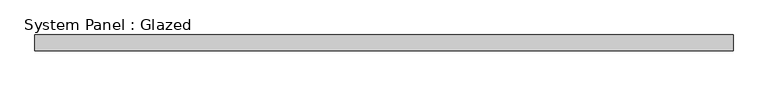
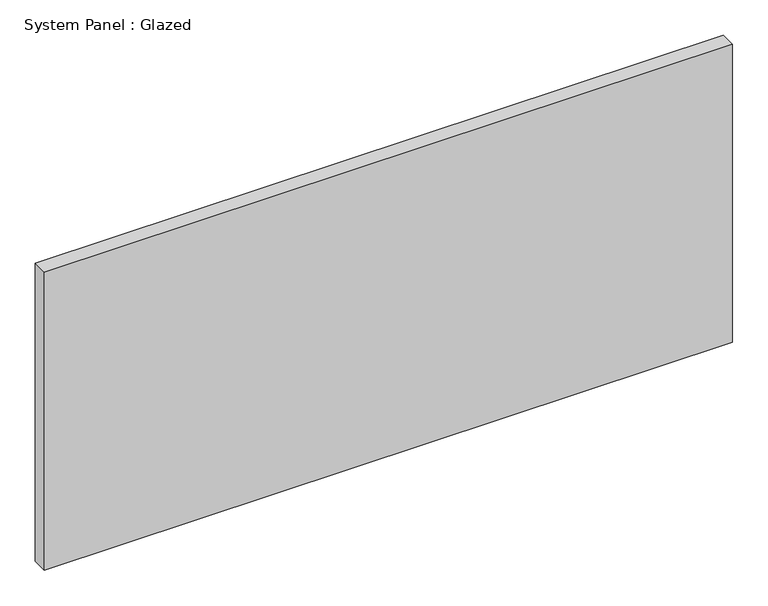
"""IFC4 building model written with IfcOpenShell, lengths in millimetres: plate geometry, System Panel : Glazed."""

from ifc_helpers import new_model, si_unit, origin, origin_with_axes, place, context, project, spatial, polyline, outline, extrude, source, transform, mapped, element, save


def system_panel_glazed_80d043f3(model_context):
    return source(origin(), model_context, "Body", "SweptSolid", [
        extrude(outline(polyline([(561.975, 19.05), (-561.975, 19.05), (-561.975, 44.45), (561.975, 44.45), (561.975, 19.05)])), origin_with_axes(), (0.0, 0.0, 1.0), 514.35),
    ])


if __name__ == "__main__":
    model = new_model("IFC4")
    model_context = context("Model", 3, world=origin())
    ifc_project = project(units=[si_unit("LENGTHUNIT", "METRE", prefix="MILLI")], contexts=[model_context])
    site = spatial("IfcSite", under=ifc_project)
    building = spatial("IfcBuilding", under=site)
    placement = place(None, origin())
    system_panel_glazed_shape = system_panel_glazed_80d043f3(model_context)
    element("IfcPlate", 1, ObjectType="System Panel : Glazed", at=placement, inside=building, context=model_context, shape_type="MappedRepresentation", body=[
        mapped(system_panel_glazed_shape, transform((0.0, 0.0, 0.0), x_axis=(1.0, 0.0, 0.0), y_axis=(0.0, 1.0, 0.0), z_axis=(0.0, 0.0, 1.0))),
    ])
    save(model, "model.ifc")

# Revit data of these elements
# Type "System Panel : Glazed"
#   Construction Type Id = "GSP4R"
#   Analytic Construction = "1/8 in Pilkington single glazing"
#   Visual Light Transmittance = 0.9
#   Solar Heat Gain Coefficient = 0.86
#   Heat Transfer Coefficient (U) = 1.18115 BTU/(h·ft²·°F)
# Element 1 (IfcPlate, "System Panel : Glazed")
#   Materials on its faces: "Glass"
# Materials
#   "Glass": class "Glass", colour RGB 0 128 192, transparency 0.75, Description = "Soda Lime Glass", Cost = 0
